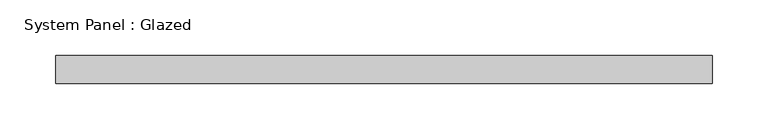
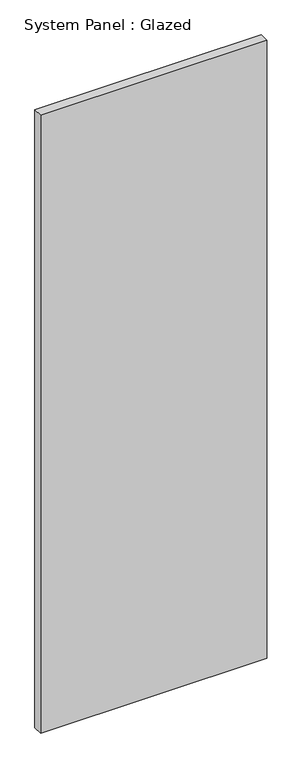
"""IFC4 building model written with IfcOpenShell, lengths in millimetres: plate geometry, System Panel : Glazed."""

from ifc_helpers import new_model, si_unit, origin, origin_with_axes, place, context, project, spatial, polyline, outline, extrude, source, transform, mapped, element, save


def system_panel_glazed_e97abd02(model_context):
    return source(origin(), model_context, "Body", "SweptSolid", [
        extrude(outline(polyline([(294.712644, -44.45), (-294.712644, -44.45), (-294.712644, -19.05), (294.712644, -19.05), (294.712644, -44.45)])), origin_with_axes(), (0.0, 0.0, 1.0), 1701.8),
    ])


if __name__ == "__main__":
    model = new_model("IFC4")
    model_context = context("Model", 3, world=origin())
    ifc_project = project(units=[si_unit("LENGTHUNIT", "METRE", prefix="MILLI")], contexts=[model_context])
    site = spatial("IfcSite", under=ifc_project)
    building = spatial("IfcBuilding", under=site)
    placement = place(None, origin())
    system_panel_glazed_shape = system_panel_glazed_e97abd02(model_context)
    element("IfcPlate", 1, ObjectType="System Panel : Glazed", at=placement, inside=building, context=model_context, shape_type="MappedRepresentation", body=[
        mapped(system_panel_glazed_shape, transform((0.0, 0.0, 0.0), x_axis=(1.0, 0.0, 0.0), y_axis=(0.0, 1.0, 0.0), z_axis=(0.0, 0.0, 1.0))),
    ])
    save(model, "model.ifc")

# Revit data of these elements
# Type "System Panel : Glazed"
#   Construction Type Id = "GSP4R"
#   Analytic Construction = "1/8 in Pilkington single glazing"
#   Visual Light Transmittance = 0.9
#   Solar Heat Gain Coefficient = 0.86
#   Heat Transfer Coefficient (U) = 1.18115 BTU/(h·ft²·°F)
#   Define Thermal Properties by = 1
# Element 1 (IfcPlate, "System Panel : Glazed")
#   Materials on its faces: "Glass"
# Materials
#   "Glass": class "Glass", colour RGB 0 128 192, transparency 0.75, Description = "Soda Lime Glass", Cost = 0
